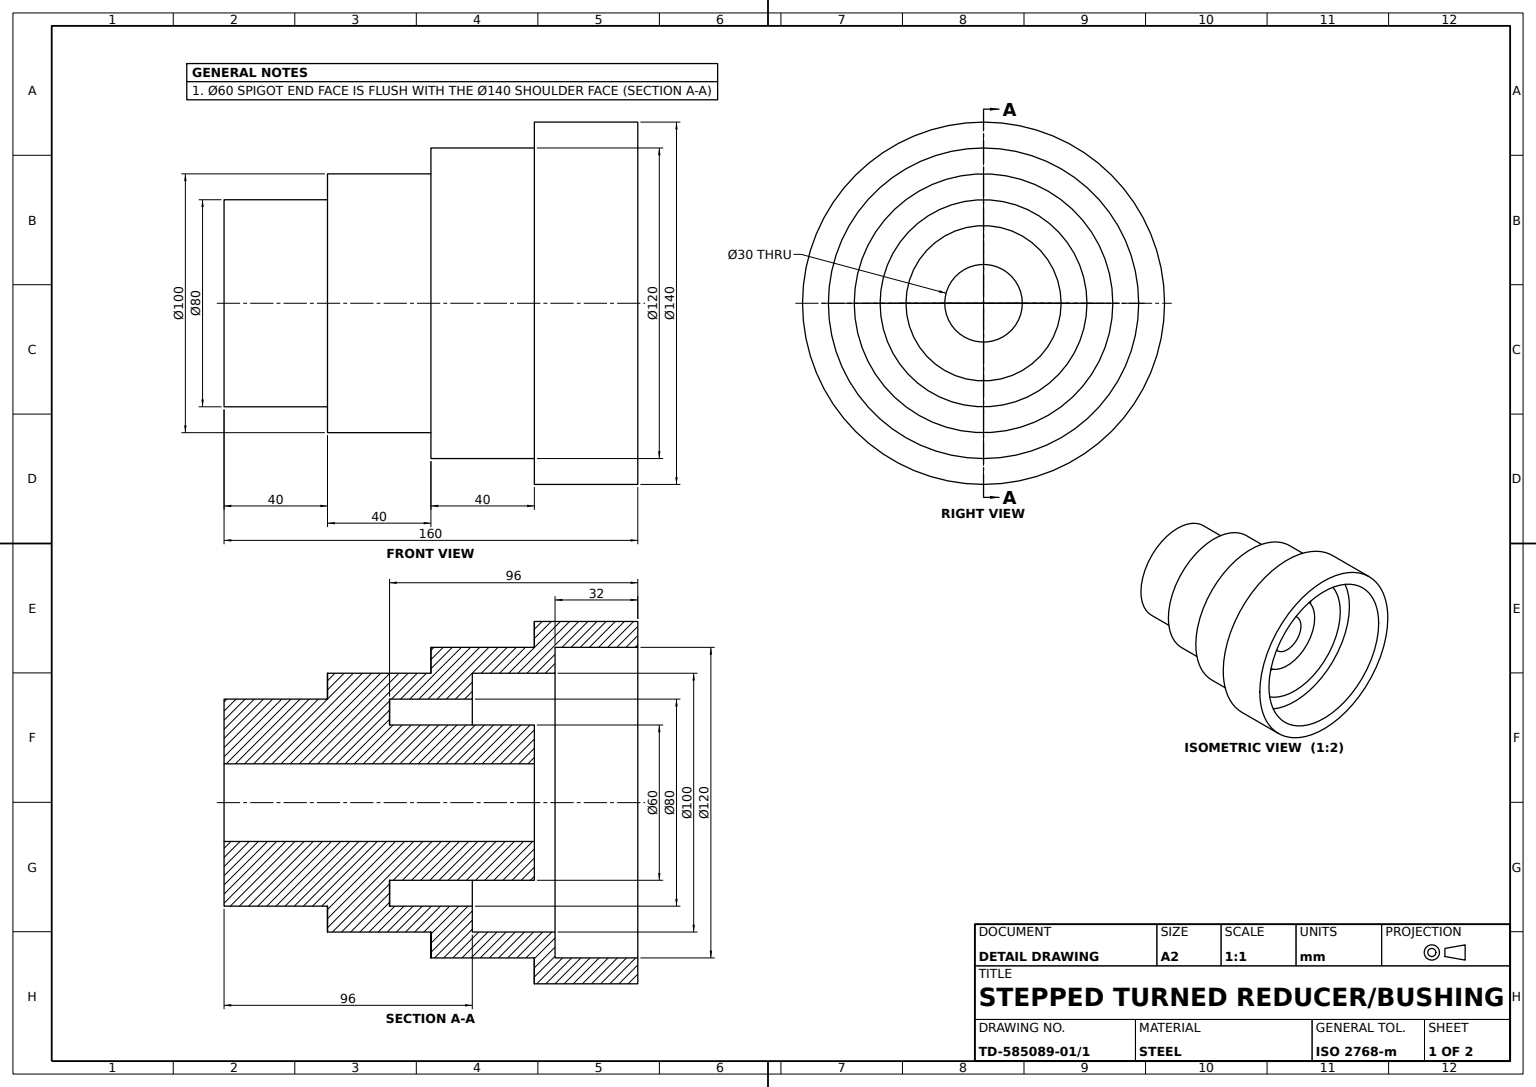
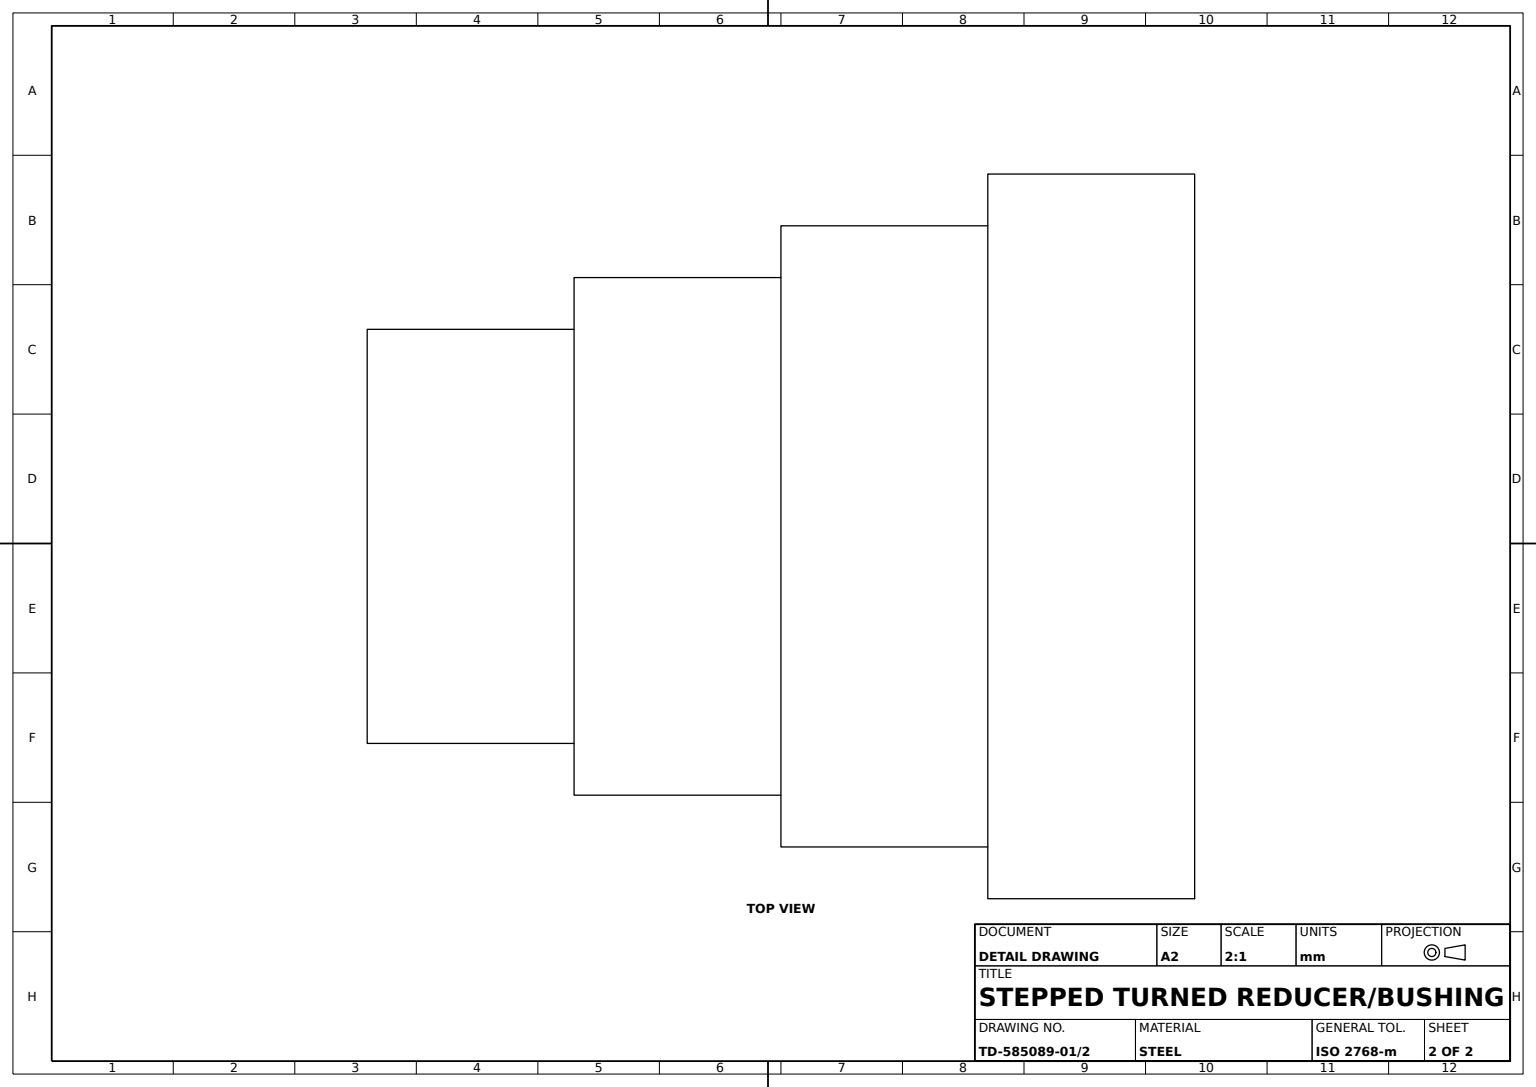
from build123d import *


with BuildPart() as part:
    # Stepped Bushing Profile → Stepped Bushing Revolve (revolve)
    with BuildSketch(Plane.XY, mode=Mode.PRIVATE) as stepped_bushing_revolve_sk:
        Polygon((-42.407900521, 15), (-42.407900521, 40), (-2.407900521, 40), (-2.407900521, 50), (37.592099479, 50), (37.592099479, 60), (77.592099479, 60), (77.592099479, 70), (117.592099479, 70), (117.592099479, 60), (85.592099479, 60), (85.592099479, 50), (53.592099479, 50), (53.592099479, 40), (21.592099479, 40), (21.592099479, 30), (77.592099479, 30), (77.592099479, 15), align=None)
    revolve(stepped_bushing_revolve_sk.sketch.rotate(Axis((-96.985663619, 0, 0), (1, 0, 0)), 90), axis=Axis((-96.985663619, 0, 0), (1, 0, 0)))


solid = part.part
